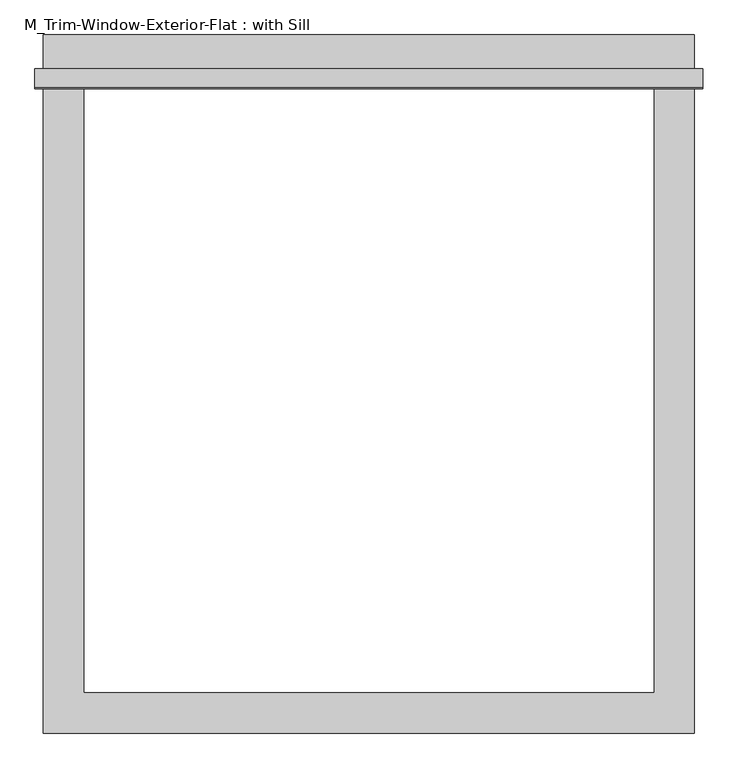
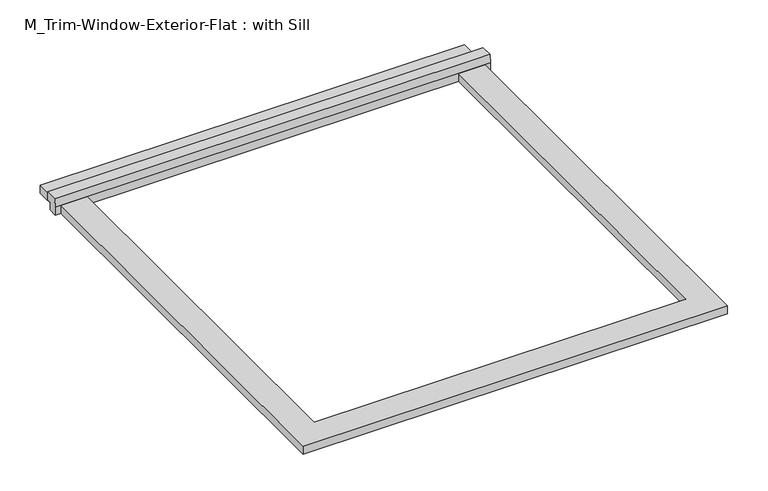
"""IFC4 building model written with IfcOpenShell, lengths in millimetres: proxy geometry, M_Trim-Window-Exterior-Flat : with Sill."""

from ifc_helpers import new_model, si_unit, frame, origin, origin_with_axes, place, context, project, spatial, polyline, outline, extrude, source, transform, mapped, element, save


def m_trim_window_exterior_flat_with_sill_c06b807c(model_context):
    return source(origin(), model_context, "Body", "SweptSolid", [
        extrude(outline(polyline([(485.0, 920.4323709), (-485.0, 920.4323709), (-485.0, 980.4323709), (485.0, 980.4323709), (485.0, 920.4323709)])), origin_with_axes(), (0.0, 0.0, 1.0), 19.05),
        extrude(outline(polyline([(930.0, 38.1), (930.0, 19.05), (920.4323709, 19.05), (920.4323709, 0.0), (900.0, 0.0), (900.0, 19.05), (902.4580645, 38.1), (930.0, 38.1)])), frame((-497.7, 0.0, 0.0), z_axis=(1.0, 0.0, 0.0), x_axis=(0.0, 1.0, 0.0)), (0.0, 0.0, 1.0), 995.4),
        extrude(outline(polyline([(-485.0, -60.0), (-485.0, 900.0), (-425.0, 900.0), (-425.0, 0.0), (425.0, 0.0), (425.0, 900.0), (485.0, 900.0), (485.0, -60.0), (-485.0, -60.0)])), origin_with_axes(), (0.0, 0.0, 1.0), 19.05),
    ])


if __name__ == "__main__":
    model = new_model("IFC4")
    model_context = context("Model", 3, world=origin())
    ifc_project = project(units=[si_unit("LENGTHUNIT", "METRE", prefix="MILLI")], contexts=[model_context])
    site = spatial("IfcSite", under=ifc_project)
    building = spatial("IfcBuilding", under=site)
    placement = place(None, origin())
    m_trim_window_exterior_flat_with_sill_shape = m_trim_window_exterior_flat_with_sill_c06b807c(model_context)
    element("IfcBuildingElementProxy", 1, Name="M_Trim-Window-Exterior-Flat : with Sill", ObjectType="M_Trim-Window-Exterior-Flat : with Sill", at=placement, inside=building, context=model_context, shape_type="MappedRepresentation", body=[
        mapped(m_trim_window_exterior_flat_with_sill_shape, transform((0.0, 0.0, 0.0), x_axis=(1.0, 0.0, 0.0), y_axis=(0.0, 1.0, 0.0), z_axis=(0.0, 0.0, 1.0))),
    ])
    save(model, "model.ifc")

# Revit data of these elements
# Type "M_Trim-Window-Exterior-Flat : with Sill"
#   Trim Width = 60 mm
#   Trim Thickness_Picture Frame = 30 mm
#   Trim Thickness_with Sill = 19.05 mm
#   Sill Thickness = 30 mm
#   Opening Width [instance default] = 600 mm
#   Opening Height [instance default] = 900 mm
#   Default Elevation = 1200 mm
#   Sill = yes
#   Picture Frame = no
#   Trim Material [instance default] = none
# Element 1 (IfcBuildingElementProxy, "M_Trim-Window-Exterior-Flat : with Sill")
#   Opening Width = 850 mm
#   Trim Material = Clad - White
#   Materials on its faces: "Clad - White"
# Materials
#   "Clad - White": class "Wood", colour RGB 242 242 238, transparency 0, Cost = 0
